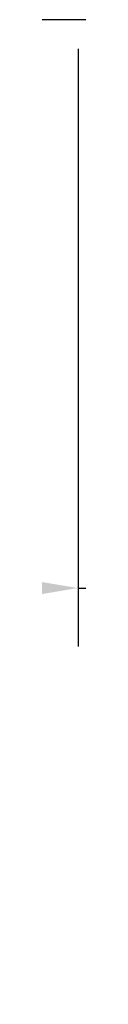
# Model space of a CAD drawing. Units: inches. Extents: x 2091 to 2899, y 967 to 2217.
# Tile 107 of 256: x 2202.51 to 2203.12, y 1131.25 to 1152.25. Entities that reach past the tile are written whole.
import ezdxf

# ---------------------------------------------------------------- set-up
doc = ezdxf.new("R2010")
doc.units = ezdxf.units.IN
doc.layers.add('A-ANNO-DIMS', color=2, linetype='Continuous', lineweight=18)
doc.styles.get("Standard").update_dxf_attribs({"font": 'arial.ttf'})
doc.dimstyles.new('ISO-25', dxfattribs={"dimtxt": 4, "dimasz": 4, "dimexe": 1.25, "dimexo": 0.625, "dimtad": 1, "dimdec": 0, "dimlunit": 3, "dimtxsty": 'Standard', "dimcen": 2.5, "dimadec": 0, "dimazin": 0, "dimtfac": 1, "dimtdec": 0, "dimtmove": 0, "dimatfit": 3, "dimfxl": 1, "dimarcsym": 0})

# ---------------------------------------------------------------- blocks, each defined once
blk = doc.blocks.new('*D37')
at = {"layer": 'A-ANNO-DIMS', "color": 0, "lineweight": -2, "transparency": 16777216}
for p, q in [((2203.116, 1151.622), (2203.116, 1138.874)), ((2212.276, 1151.622), (2212.276, 1138.874)), ((2199.116, 1140.124), (2195.116, 1140.124)), ((2203.116, 1140.124), (2212.276, 1140.124)), ((2216.276, 1140.124), (2245.908, 1140.124))]:
    blk.add_line(p, q, dxfattribs=at)
at = {"layer": 'A-ANNO-DIMS', "color": 0, "transparency": 16777216}
for points in [[(2199.116, 1140.79), (2199.116, 1139.457), (2203.116, 1140.124)], [(2216.276, 1140.79), (2216.276, 1139.457), (2212.276, 1140.124)]]:
    blk.add_solid(points, dxfattribs=at)
at = {"layer": 'Defpoints', "color": 0, "transparency": 16777216}
for p in [(2203.116, 1152.247), (2212.276, 1152.247), (2212.276, 1140.124)]:
    blk.add_point(p, dxfattribs=at)
at = {"layer": 'A-ANNO-DIMS', "color": 0, "transparency": 16777216, "insert": (2233.092, 1142.791), "char_height": 4, "attachment_point": 5}
blk.add_mtext('0\'-9" TYP.', dxfattribs=at)
blk = doc.blocks.new('*D91')
at = {"layer": 'A-ANNO-DIMS', "color": 0, "lineweight": -2, "transparency": 16777216}
for p, q in [((2211.651, 1152.247), (2098.311, 1152.247)), ((2099.561, 1103.919), (2099.561, 1148.247)), ((2211.519, 1099.919), (2098.311, 1099.919))]:
    blk.add_line(p, q, dxfattribs=at)
at = {"layer": 'A-ANNO-DIMS', "color": 0, "transparency": 16777216}
for points in [[(2098.895, 1148.247), (2100.228, 1148.247), (2099.561, 1152.247)], [(2098.895, 1103.919), (2100.228, 1103.919), (2099.561, 1099.919)]]:
    blk.add_solid(points, dxfattribs=at)
at = {"layer": 'Defpoints', "color": 0, "transparency": 16777216}
for p in [(2099.561, 1152.247), (2212.276, 1152.247), (2212.144, 1099.919)]:
    blk.add_point(p, dxfattribs=at)
at = {"layer": 'A-ANNO-DIMS', "color": 0, "transparency": 16777216, "insert": (2096.868, 1126.083), "char_height": 4, "attachment_point": 5, "rotation": 90}
blk.add_mtext('4\'-4 1/2"', dxfattribs=at)

msp = doc.modelspace()

# ---------------------------------------------------------------- dimensions: what is measured, and where the dimension line sits
at = {"layer": 'A-ANNO-DIMS'}
dim = msp.add_linear_dim(base=(2099.561, 1152.247), p1=(2212.144, 1099.919), p2=(2212.276, 1152.247), angle=90, dimstyle='ISO-25', override={"dimdec": 1, "dimlfac": 1, "dimrnd": 0, "dimzin": 1, "dimdsep": 46, "dimlunit": 4, "dimfrac": 2}, dxfattribs=at)
dim.commit()
dim.dimension.update_dxf_attribs({"geometry": '*D91', "text_midpoint": (2096.868, 1126.083)})
dim = msp.add_linear_dim(base=(2212.276, 1140.124), p1=(2203.116, 1152.247), p2=(2212.276, 1152.247), text='<> TYP.', dimstyle='ISO-25', override={"dimdec": 1, "dimlfac": 1, "dimrnd": 0, "dimzin": 1, "dimdsep": 46, "dimlunit": 4, "dimfrac": 2}, dxfattribs=at)
dim.commit()
dim.dimension.update_dxf_attribs({"geometry": '*D37', "text_midpoint": (2233.092, 1142.791)})

doc.saveas('drawing.dxf')
